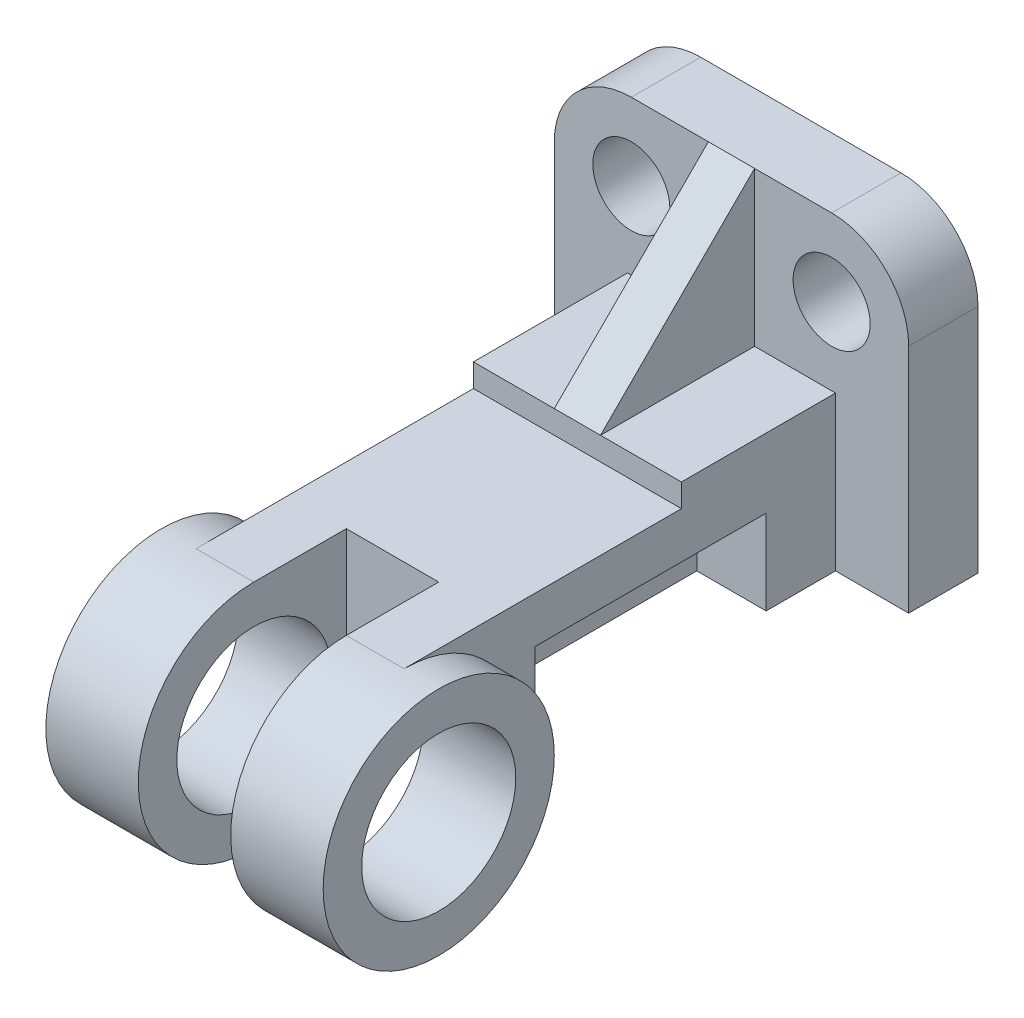
ISO-10303-21;
HEADER;
FILE_DESCRIPTION(('STEP AP214'),'2;1');
FILE_NAME('part.step','',(''),(''),'','','');
FILE_SCHEMA(('AUTOMOTIVE_DESIGN { 1 0 10303 214 1 1 1 1 }'));
ENDSEC;
DATA;
#1=APPLICATION_CONTEXT('core data for automotive mechanical design processes');
#2=APPLICATION_PROTOCOL_DEFINITION('international standard','automotive_design',2000,#1);
#3=PRODUCT_CONTEXT('',#1,'mechanical');
#4=PRODUCT('Part','Part','',(#3));
#5=PRODUCT_RELATED_PRODUCT_CATEGORY('part','',(#4));
#6=PRODUCT_DEFINITION_FORMATION('','',#4);
#7=PRODUCT_DEFINITION_CONTEXT('part definition',#1,'design');
#8=PRODUCT_DEFINITION('design','',#6,#7);
#9=PRODUCT_DEFINITION_SHAPE('','',#8);
#10=(LENGTH_UNIT() NAMED_UNIT(*) SI_UNIT(.MILLI.,.METRE.));
#11=(NAMED_UNIT(*) PLANE_ANGLE_UNIT() SI_UNIT($,.RADIAN.));
#12=(NAMED_UNIT(*) SI_UNIT($,.STERADIAN.) SOLID_ANGLE_UNIT());
#13=UNCERTAINTY_MEASURE_WITH_UNIT(LENGTH_MEASURE(1.E-05),#10,'distance_accuracy_value','');
#14=(GEOMETRIC_REPRESENTATION_CONTEXT(3) GLOBAL_UNCERTAINTY_ASSIGNED_CONTEXT((#13)) GLOBAL_UNIT_ASSIGNED_CONTEXT((#10,
#11,#12)) REPRESENTATION_CONTEXT('',''));
#15=CARTESIAN_POINT('',(0.,0.,0.));
#16=DIRECTION('',(0.,0.,1.));
#17=DIRECTION('',(1.,0.,0.));
#18=AXIS2_PLACEMENT_3D('',#15,#16,#17);
#19=CARTESIAN_POINT('',(0.,0.,106.));
#20=DIRECTION('',(0.,0.,1.));
#21=DIRECTION('',(1.,0.,0.));
#22=AXIS2_PLACEMENT_3D('',#19,#20,#21);
#23=PLANE('',#22);
#24=DIRECTION('',(1.,0.,0.));
#25=VECTOR('',#24,1.);
#26=CARTESIAN_POINT('',(0.,34.,106.));
#27=LINE('',#26,#25);
#28=CARTESIAN_POINT('',(34.,34.,106.));
#29=VERTEX_POINT('',#28);
#30=CARTESIAN_POINT('',(58.,34.,106.));
#31=VERTEX_POINT('',#30);
#32=EDGE_CURVE('E66',#29,#31,#27,.T.);
#33=ORIENTED_EDGE('',*,*,#32,.F.);
#34=DIRECTION('',(0.,-1.,0.));
#35=VECTOR('',#34,1.);
#36=CARTESIAN_POINT('',(34.,0.,106.));
#37=LINE('',#36,#35);
#38=CARTESIAN_POINT('',(34.,0.,106.));
#39=VERTEX_POINT('',#38);
#40=EDGE_CURVE('E256',#29,#39,#37,.T.);
#41=ORIENTED_EDGE('',*,*,#40,.T.);
#42=DIRECTION('',(1.,0.,0.));
#43=VECTOR('',#42,1.);
#44=CARTESIAN_POINT('',(0.,0.,106.));
#45=LINE('',#44,#43);
#46=CARTESIAN_POINT('',(58.,0.,106.));
#47=VERTEX_POINT('',#46);
#48=EDGE_CURVE('E355',#39,#47,#45,.T.);
#49=ORIENTED_EDGE('',*,*,#48,.T.);
#50=DIRECTION('',(0.,1.,0.));
#51=VECTOR('',#50,1.);
#52=CARTESIAN_POINT('',(58.,0.,106.));
#53=LINE('',#52,#51);
#54=EDGE_CURVE('E245',#47,#31,#53,.T.);
#55=ORIENTED_EDGE('',*,*,#54,.T.);
#56=EDGE_LOOP('',(#33,#41,#49,#55));
#57=FACE_BOUND('',#56,.T.);
#58=ADVANCED_FACE('F43',(#57),#23,.T.);
#59=CARTESIAN_POINT('',(10.,4.00000000000001,130.));
#60=DIRECTION('',(1.,0.,0.));
#61=DIRECTION('',(0.,0.,-1.));
#62=AXIS2_PLACEMENT_3D('',#59,#60,#61);
#63=CYLINDRICAL_SURFACE('',#62,30.);
#64=CARTESIAN_POINT('',(10.,4.00000000000001,130.));
#65=DIRECTION('',(1.,0.,0.));
#66=DIRECTION('',(0.,0.,-1.));
#67=AXIS2_PLACEMENT_3D('',#64,#65,#66);
#68=CIRCLE('',#67,30.);
#69=CARTESIAN_POINT('',(10.,4.00000000000001,100.));
#70=VERTEX_POINT('',#69);
#71=EDGE_CURVE('E251',#70,#70,#68,.T.);
#72=ORIENTED_EDGE('',*,*,#71,.T.);
#73=EDGE_LOOP('',(#72));
#74=FACE_BOUND('',#73,.T.);
#75=CARTESIAN_POINT('',(34.,4.00000000000001,130.));
#76=DIRECTION('',(1.,0.,0.));
#77=DIRECTION('',(0.,0.,-1.));
#78=AXIS2_PLACEMENT_3D('',#75,#76,#77);
#79=CIRCLE('',#78,30.);
#80=CARTESIAN_POINT('',(34.,34.,130.));
#81=VERTEX_POINT('',#80);
#82=CARTESIAN_POINT('',(34.,0.,100.267862505363));
#83=VERTEX_POINT('',#82);
#84=EDGE_CURVE('E242',#81,#83,#79,.T.);
#85=ORIENTED_EDGE('',*,*,#84,.F.);
#86=DIRECTION('',(1.,0.,0.));
#87=VECTOR('',#86,1.);
#88=CARTESIAN_POINT('',(19.,34.,130.));
#89=LINE('',#88,#87);
#90=CARTESIAN_POINT('',(19.,34.,130.));
#91=VERTEX_POINT('',#90);
#92=EDGE_CURVE('E228',#91,#81,#89,.T.);
#93=ORIENTED_EDGE('',*,*,#92,.F.);
#94=CARTESIAN_POINT('',(19.,4.00000000000001,130.));
#95=DIRECTION('',(1.,0.,0.));
#96=DIRECTION('',(0.,0.,-1.));
#97=AXIS2_PLACEMENT_3D('',#94,#95,#96);
#98=CIRCLE('',#97,30.);
#99=CARTESIAN_POINT('',(19.,0.,100.267862505363));
#100=VERTEX_POINT('',#99);
#101=EDGE_CURVE('E55',#100,#91,#98,.T.);
#102=ORIENTED_EDGE('',*,*,#101,.F.);
#103=DIRECTION('',(1.,0.,0.));
#104=VECTOR('',#103,1.);
#105=CARTESIAN_POINT('',(10.,0.,100.267862505363));
#106=LINE('',#105,#104);
#107=EDGE_CURVE('E258',#83,#100,#106,.F.);
#108=ORIENTED_EDGE('',*,*,#107,.F.);
#109=EDGE_LOOP('',(#85,#93,#102,#108));
#110=FACE_BOUND('',#109,.T.);
#111=ADVANCED_FACE('F243',(#74,#110),#63,.T.);
#112=CARTESIAN_POINT('',(0.,0.,18.));
#113=DIRECTION('',(0.,1.,0.));
#114=DIRECTION('',(0.,0.,1.));
#115=AXIS2_PLACEMENT_3D('',#112,#113,#114);
#116=PLANE('',#115);
#117=DIRECTION('',(0.,0.,1.));
#118=VECTOR('',#117,1.);
#119=CARTESIAN_POINT('',(34.,0.,18.));
#120=LINE('',#119,#118);
#121=EDGE_CURVE('E11',#83,#39,#120,.T.);
#122=ORIENTED_EDGE('',*,*,#121,.F.);
#123=ORIENTED_EDGE('',*,*,#107,.T.);
#124=DIRECTION('',(0.,0.,-1.));
#125=VECTOR('',#124,1.);
#126=CARTESIAN_POINT('',(19.,0.,106.));
#127=LINE('',#126,#125);
#128=CARTESIAN_POINT('',(19.,0.,96.));
#129=VERTEX_POINT('',#128);
#130=EDGE_CURVE('E238',#100,#129,#127,.T.);
#131=ORIENTED_EDGE('',*,*,#130,.T.);
#132=DIRECTION('',(-1.,0.,0.));
#133=VECTOR('',#132,1.);
#134=CARTESIAN_POINT('',(37.,0.,96.));
#135=LINE('',#134,#133);
#136=CARTESIAN_POINT('',(37.,0.,96.));
#137=VERTEX_POINT('',#136);
#138=EDGE_CURVE('E304',#137,#129,#135,.T.);
#139=ORIENTED_EDGE('',*,*,#138,.F.);
#140=DIRECTION('',(0.,0.,1.));
#141=VECTOR('',#140,1.);
#142=CARTESIAN_POINT('',(37.,0.,0.));
#143=LINE('',#142,#141);
#144=CARTESIAN_POINT('',(37.,0.,36.));
#145=VERTEX_POINT('',#144);
#146=EDGE_CURVE('E294',#145,#137,#143,.T.);
#147=ORIENTED_EDGE('',*,*,#146,.F.);
#148=DIRECTION('',(-1.,0.,0.));
#149=VECTOR('',#148,1.);
#150=CARTESIAN_POINT('',(37.,0.,36.));
#151=LINE('',#150,#149);
#152=CARTESIAN_POINT('',(19.,0.,36.));
#153=VERTEX_POINT('',#152);
#154=EDGE_CURVE('E307',#145,#153,#151,.T.);
#155=ORIENTED_EDGE('',*,*,#154,.T.);
#156=CARTESIAN_POINT('',(19.,0.,18.));
#157=VERTEX_POINT('',#156);
#158=EDGE_CURVE('E351',#153,#157,#127,.T.);
#159=ORIENTED_EDGE('',*,*,#158,.T.);
#160=DIRECTION('',(1.,0.,0.));
#161=VECTOR('',#160,1.);
#162=CARTESIAN_POINT('',(0.,0.,18.));
#163=LINE('',#162,#161);
#164=CARTESIAN_POINT('',(0.,0.,18.));
#165=VERTEX_POINT('',#164);
#166=EDGE_CURVE('E401',#165,#157,#163,.T.);
#167=ORIENTED_EDGE('',*,*,#166,.F.);
#168=DIRECTION('',(0.,0.,-1.));
#169=VECTOR('',#168,1.);
#170=CARTESIAN_POINT('',(0.,0.,18.));
#171=LINE('',#170,#169);
#172=CARTESIAN_POINT('',(0.,0.,0.));
#173=VERTEX_POINT('',#172);
#174=EDGE_CURVE('E425',#165,#173,#171,.T.);
#175=ORIENTED_EDGE('',*,*,#174,.T.);
#176=DIRECTION('',(1.,0.,0.));
#177=VECTOR('',#176,1.);
#178=CARTESIAN_POINT('',(0.,0.,0.));
#179=LINE('',#178,#177);
#180=CARTESIAN_POINT('',(92.,0.,0.));
#181=VERTEX_POINT('',#180);
#182=EDGE_CURVE('E414',#173,#181,#179,.T.);
#183=ORIENTED_EDGE('',*,*,#182,.T.);
#184=DIRECTION('',(0.,0.,-1.));
#185=VECTOR('',#184,1.);
#186=CARTESIAN_POINT('',(92.,0.,18.));
#187=LINE('',#186,#185);
#188=CARTESIAN_POINT('',(92.,0.,18.));
#189=VERTEX_POINT('',#188);
#190=EDGE_CURVE('E413',#189,#181,#187,.T.);
#191=ORIENTED_EDGE('',*,*,#190,.F.);
#192=CARTESIAN_POINT('',(73.,0.,18.));
#193=VERTEX_POINT('',#192);
#194=EDGE_CURVE('E402',#193,#189,#163,.T.);
#195=ORIENTED_EDGE('',*,*,#194,.F.);
#196=DIRECTION('',(0.,0.,-1.));
#197=VECTOR('',#196,1.);
#198=CARTESIAN_POINT('',(73.,0.,106.));
#199=LINE('',#198,#197);
#200=CARTESIAN_POINT('',(73.,0.,36.));
#201=VERTEX_POINT('',#200);
#202=EDGE_CURVE('E367',#201,#193,#199,.T.);
#203=ORIENTED_EDGE('',*,*,#202,.F.);
#204=DIRECTION('',(1.,0.,0.));
#205=VECTOR('',#204,1.);
#206=CARTESIAN_POINT('',(55.,0.,36.));
#207=LINE('',#206,#205);
#208=CARTESIAN_POINT('',(55.,0.,36.));
#209=VERTEX_POINT('',#208);
#210=EDGE_CURVE('E341',#209,#201,#207,.T.);
#211=ORIENTED_EDGE('',*,*,#210,.F.);
#212=DIRECTION('',(0.,0.,-1.));
#213=VECTOR('',#212,1.);
#214=CARTESIAN_POINT('',(55.,0.,0.));
#215=LINE('',#214,#213);
#216=CARTESIAN_POINT('',(55.,0.,96.));
#217=VERTEX_POINT('',#216);
#218=EDGE_CURVE('E329',#217,#209,#215,.T.);
#219=ORIENTED_EDGE('',*,*,#218,.F.);
#220=DIRECTION('',(1.,0.,0.));
#221=VECTOR('',#220,1.);
#222=CARTESIAN_POINT('',(55.,0.,96.));
#223=LINE('',#222,#221);
#224=CARTESIAN_POINT('',(73.,0.,96.));
#225=VERTEX_POINT('',#224);
#226=EDGE_CURVE('E350',#217,#225,#223,.T.);
#227=ORIENTED_EDGE('',*,*,#226,.T.);
#228=CARTESIAN_POINT('',(73.,0.,100.267862505363));
#229=VERTEX_POINT('',#228);
#230=EDGE_CURVE('E369',#229,#225,#199,.T.);
#231=ORIENTED_EDGE('',*,*,#230,.F.);
#232=DIRECTION('',(-1.,0.,0.));
#233=VECTOR('',#232,1.);
#234=CARTESIAN_POINT('',(82.,0.,100.267862505363));
#235=LINE('',#234,#233);
#236=CARTESIAN_POINT('',(58.,0.,100.267862505363));
#237=VERTEX_POINT('',#236);
#238=EDGE_CURVE('E284',#237,#229,#235,.F.);
#239=ORIENTED_EDGE('',*,*,#238,.F.);
#240=DIRECTION('',(0.,0.,-1.));
#241=VECTOR('',#240,1.);
#242=CARTESIAN_POINT('',(58.,0.,18.));
#243=LINE('',#242,#241);
#244=EDGE_CURVE('E278',#47,#237,#243,.T.);
#245=ORIENTED_EDGE('',*,*,#244,.F.);
#246=ORIENTED_EDGE('',*,*,#48,.F.);
#247=EDGE_LOOP('',(#122,#123,#131,#139,#147,#155,#159,#167,#175,#183,#191,#195,#203,#211,#219,
#227,#231,#239,#245,#246));
#248=FACE_BOUND('',#247,.T.);
#249=ADVANCED_FACE('F471',(#248),#116,.F.);
#250=CARTESIAN_POINT('',(19.,0.,106.));
#251=DIRECTION('',(1.,0.,0.));
#252=DIRECTION('',(0.,0.,-1.));
#253=AXIS2_PLACEMENT_3D('',#250,#251,#252);
#254=PLANE('',#253);
#255=ORIENTED_EDGE('',*,*,#130,.F.);
#256=ORIENTED_EDGE('',*,*,#101,.T.);
#257=DIRECTION('',(0.,0.,-1.));
#258=VECTOR('',#257,1.);
#259=CARTESIAN_POINT('',(19.,34.,106.));
#260=LINE('',#259,#258);
#261=CARTESIAN_POINT('',(19.,34.,58.));
#262=VERTEX_POINT('',#261);
#263=EDGE_CURVE('E225',#91,#262,#260,.T.);
#264=ORIENTED_EDGE('',*,*,#263,.T.);
#265=DIRECTION('',(0.,1.,0.));
#266=VECTOR('',#265,1.);
#267=CARTESIAN_POINT('',(19.,0.,58.));
#268=LINE('',#267,#266);
#269=CARTESIAN_POINT('',(19.,40.,58.));
#270=VERTEX_POINT('',#269);
#271=EDGE_CURVE('E455',#262,#270,#268,.T.);
#272=ORIENTED_EDGE('',*,*,#271,.T.);
#273=DIRECTION('',(0.,0.,-1.));
#274=VECTOR('',#273,1.);
#275=CARTESIAN_POINT('',(19.,40.,106.));
#276=LINE('',#275,#274);
#277=CARTESIAN_POINT('',(19.,40.,18.));
#278=VERTEX_POINT('',#277);
#279=EDGE_CURVE('E362',#270,#278,#276,.T.);
#280=ORIENTED_EDGE('',*,*,#279,.T.);
#281=DIRECTION('',(0.,-1.,0.));
#282=VECTOR('',#281,1.);
#283=CARTESIAN_POINT('',(19.,0.,18.));
#284=LINE('',#283,#282);
#285=EDGE_CURVE('E353',#278,#157,#284,.T.);
#286=ORIENTED_EDGE('',*,*,#285,.T.);
#287=ORIENTED_EDGE('',*,*,#158,.F.);
#288=DIRECTION('',(0.,1.,0.));
#289=VECTOR('',#288,1.);
#290=CARTESIAN_POINT('',(19.,0.,36.));
#291=LINE('',#290,#289);
#292=CARTESIAN_POINT('',(19.,22.,36.));
#293=VERTEX_POINT('',#292);
#294=EDGE_CURVE('E293',#153,#293,#291,.T.);
#295=ORIENTED_EDGE('',*,*,#294,.T.);
#296=DIRECTION('',(0.,0.,1.));
#297=VECTOR('',#296,1.);
#298=CARTESIAN_POINT('',(19.,22.,0.));
#299=LINE('',#298,#297);
#300=CARTESIAN_POINT('',(19.,22.,96.));
#301=VERTEX_POINT('',#300);
#302=EDGE_CURVE('E297',#293,#301,#299,.T.);
#303=ORIENTED_EDGE('',*,*,#302,.T.);
#304=DIRECTION('',(0.,-1.,0.));
#305=VECTOR('',#304,1.);
#306=CARTESIAN_POINT('',(19.,0.,96.));
#307=LINE('',#306,#305);
#308=EDGE_CURVE('E290',#301,#129,#307,.T.);
#309=ORIENTED_EDGE('',*,*,#308,.T.);
#310=EDGE_LOOP('',(#255,#256,#264,#272,#280,#286,#287,#295,#303,#309));
#311=FACE_BOUND('',#310,.T.);
#312=ADVANCED_FACE('F236',(#311),#254,.F.);
#313=CARTESIAN_POINT('',(0.,40.,106.));
#314=DIRECTION('',(0.,1.,0.));
#315=DIRECTION('',(0.,0.,1.));
#316=AXIS2_PLACEMENT_3D('',#313,#314,#315);
#317=PLANE('',#316);
#318=DIRECTION('',(1.,0.,0.));
#319=VECTOR('',#318,1.);
#320=CARTESIAN_POINT('',(0.,40.,58.));
#321=LINE('',#320,#319);
#322=CARTESIAN_POINT('',(52.,40.,58.));
#323=VERTEX_POINT('',#322);
#324=CARTESIAN_POINT('',(73.,40.,58.));
#325=VERTEX_POINT('',#324);
#326=EDGE_CURVE('E316',#323,#325,#321,.T.);
#327=ORIENTED_EDGE('',*,*,#326,.T.);
#328=DIRECTION('',(0.,0.,-1.));
#329=VECTOR('',#328,1.);
#330=CARTESIAN_POINT('',(73.,40.,106.));
#331=LINE('',#330,#329);
#332=CARTESIAN_POINT('',(73.,40.,18.));
#333=VERTEX_POINT('',#332);
#334=EDGE_CURVE('E370',#325,#333,#331,.T.);
#335=ORIENTED_EDGE('',*,*,#334,.T.);
#336=DIRECTION('',(1.,0.,0.));
#337=VECTOR('',#336,1.);
#338=CARTESIAN_POINT('',(0.,40.,18.));
#339=LINE('',#338,#337);
#340=CARTESIAN_POINT('',(52.,40.,18.));
#341=VERTEX_POINT('',#340);
#342=EDGE_CURVE('E356',#341,#333,#339,.T.);
#343=ORIENTED_EDGE('',*,*,#342,.F.);
#344=DIRECTION('',(0.,0.,-1.));
#345=VECTOR('',#344,1.);
#346=CARTESIAN_POINT('',(52.,40.,58.));
#347=LINE('',#346,#345);
#348=EDGE_CURVE('E384',#323,#341,#347,.T.);
#349=ORIENTED_EDGE('',*,*,#348,.F.);
#350=EDGE_LOOP('',(#327,#335,#343,#349));
#351=FACE_BOUND('',#350,.T.);
#352=ADVANCED_FACE('F505',(#351),#317,.T.);
#353=CARTESIAN_POINT('',(0.,0.,18.));
#354=DIRECTION('',(0.,0.,1.));
#355=DIRECTION('',(1.,0.,0.));
#356=AXIS2_PLACEMENT_3D('',#353,#354,#355);
#357=PLANE('',#356);
#358=CARTESIAN_POINT('',(72.,60.,18.));
#359=DIRECTION('',(0.,0.,1.));
#360=DIRECTION('',(1.,0.,0.));
#361=AXIS2_PLACEMENT_3D('',#358,#359,#360);
#362=CIRCLE('',#361,9.99999999999999);
#363=CARTESIAN_POINT('',(82.,60.,18.));
#364=VERTEX_POINT('',#363);
#365=EDGE_CURVE('E391',#364,#364,#362,.T.);
#366=ORIENTED_EDGE('',*,*,#365,.F.);
#367=EDGE_LOOP('',(#366));
#368=FACE_BOUND('',#367,.T.);
#369=ORIENTED_EDGE('',*,*,#342,.T.);
#370=DIRECTION('',(0.,1.,0.));
#371=VECTOR('',#370,1.);
#372=CARTESIAN_POINT('',(73.,0.,18.));
#373=LINE('',#372,#371);
#374=EDGE_CURVE('E345',#193,#333,#373,.T.);
#375=ORIENTED_EDGE('',*,*,#374,.F.);
#376=ORIENTED_EDGE('',*,*,#194,.T.);
#377=DIRECTION('',(0.,1.,0.));
#378=VECTOR('',#377,1.);
#379=CARTESIAN_POINT('',(92.,0.,18.));
#380=LINE('',#379,#378);
#381=CARTESIAN_POINT('',(92.,60.,18.));
#382=VERTEX_POINT('',#381);
#383=EDGE_CURVE('E408',#189,#382,#380,.T.);
#384=ORIENTED_EDGE('',*,*,#383,.T.);
#385=CARTESIAN_POINT('',(72.,60.,18.));
#386=DIRECTION('',(0.,0.,1.));
#387=DIRECTION('',(1.,0.,0.));
#388=AXIS2_PLACEMENT_3D('',#385,#386,#387);
#389=CIRCLE('',#388,20.);
#390=CARTESIAN_POINT('',(72.,80.,18.));
#391=VERTEX_POINT('',#390);
#392=EDGE_CURVE('E439',#382,#391,#389,.T.);
#393=ORIENTED_EDGE('',*,*,#392,.T.);
#394=DIRECTION('',(-1.,0.,0.));
#395=VECTOR('',#394,1.);
#396=CARTESIAN_POINT('',(92.,80.,18.));
#397=LINE('',#396,#395);
#398=CARTESIAN_POINT('',(52.,80.,18.));
#399=VERTEX_POINT('',#398);
#400=EDGE_CURVE('E406',#391,#399,#397,.T.);
#401=ORIENTED_EDGE('',*,*,#400,.T.);
#402=DIRECTION('',(0.,1.,0.));
#403=VECTOR('',#402,1.);
#404=CARTESIAN_POINT('',(52.,0.,18.));
#405=LINE('',#404,#403);
#406=EDGE_CURVE('E375',#341,#399,#405,.T.);
#407=ORIENTED_EDGE('',*,*,#406,.F.);
#408=EDGE_LOOP('',(#369,#375,#376,#384,#393,#401,#407));
#409=FACE_BOUND('',#408,.T.);
#410=ADVANCED_FACE('F500',(#368,#409),#357,.T.);
#411=CARTESIAN_POINT('',(0.,80.,18.));
#412=DIRECTION('',(1.,0.,0.));
#413=DIRECTION('',(0.,0.,-1.));
#414=AXIS2_PLACEMENT_3D('',#411,#412,#413);
#415=PLANE('',#414);
#416=DIRECTION('',(0.,-1.,0.));
#417=VECTOR('',#416,1.);
#418=CARTESIAN_POINT('',(0.,80.,18.));
#419=LINE('',#418,#417);
#420=CARTESIAN_POINT('',(0.,60.,18.));
#421=VERTEX_POINT('',#420);
#422=EDGE_CURVE('E396',#421,#165,#419,.T.);
#423=ORIENTED_EDGE('',*,*,#422,.F.);
#424=DIRECTION('',(0.,0.,-1.));
#425=VECTOR('',#424,1.);
#426=CARTESIAN_POINT('',(0.,60.,18.));
#427=LINE('',#426,#425);
#428=CARTESIAN_POINT('',(0.,60.,0.));
#429=VERTEX_POINT('',#428);
#430=EDGE_CURVE('E430',#421,#429,#427,.T.);
#431=ORIENTED_EDGE('',*,*,#430,.T.);
#432=DIRECTION('',(0.,-1.,0.));
#433=VECTOR('',#432,1.);
#434=CARTESIAN_POINT('',(0.,80.,0.));
#435=LINE('',#434,#433);
#436=EDGE_CURVE('E386',#429,#173,#435,.T.);
#437=ORIENTED_EDGE('',*,*,#436,.T.);
#438=ORIENTED_EDGE('',*,*,#174,.F.);
#439=EDGE_LOOP('',(#423,#431,#437,#438));
#440=FACE_BOUND('',#439,.T.);
#441=ADVANCED_FACE('F610',(#440),#415,.F.);
#442=CARTESIAN_POINT('',(92.,0.,18.));
#443=DIRECTION('',(-1.,0.,0.));
#444=DIRECTION('',(0.,0.,1.));
#445=AXIS2_PLACEMENT_3D('',#442,#443,#444);
#446=PLANE('',#445);
#447=DIRECTION('',(0.,1.,0.));
#448=VECTOR('',#447,1.);
#449=CARTESIAN_POINT('',(92.,0.,0.));
#450=LINE('',#449,#448);
#451=CARTESIAN_POINT('',(92.,60.,0.));
#452=VERTEX_POINT('',#451);
#453=EDGE_CURVE('E420',#181,#452,#450,.T.);
#454=ORIENTED_EDGE('',*,*,#453,.T.);
#455=DIRECTION('',(0.,0.,-1.));
#456=VECTOR('',#455,1.);
#457=CARTESIAN_POINT('',(92.,60.,18.));
#458=LINE('',#457,#456);
#459=EDGE_CURVE('E443',#452,#382,#458,.F.);
#460=ORIENTED_EDGE('',*,*,#459,.T.);
#461=ORIENTED_EDGE('',*,*,#383,.F.);
#462=ORIENTED_EDGE('',*,*,#190,.T.);
#463=EDGE_LOOP('',(#454,#460,#461,#462));
#464=FACE_BOUND('',#463,.T.);
#465=ADVANCED_FACE('F602',(#464),#446,.F.);
#466=CARTESIAN_POINT('',(92.,80.,18.));
#467=DIRECTION('',(0.,-1.,0.));
#468=DIRECTION('',(0.,0.,-1.));
#469=AXIS2_PLACEMENT_3D('',#466,#467,#468);
#470=PLANE('',#469);
#471=CARTESIAN_POINT('',(40.,80.,18.));
#472=VERTEX_POINT('',#471);
#473=CARTESIAN_POINT('',(20.,80.,18.));
#474=VERTEX_POINT('',#473);
#475=EDGE_CURVE('E410',#472,#474,#397,.T.);
#476=ORIENTED_EDGE('',*,*,#475,.F.);
#477=DIRECTION('',(1.,0.,0.));
#478=VECTOR('',#477,1.);
#479=CARTESIAN_POINT('',(52.,80.,18.));
#480=LINE('',#479,#478);
#481=EDGE_CURVE('E449',#472,#399,#480,.T.);
#482=ORIENTED_EDGE('',*,*,#481,.T.);
#483=ORIENTED_EDGE('',*,*,#400,.F.);
#484=DIRECTION('',(0.,0.,-1.));
#485=VECTOR('',#484,1.);
#486=CARTESIAN_POINT('',(72.,80.,18.));
#487=LINE('',#486,#485);
#488=CARTESIAN_POINT('',(72.,80.,0.));
#489=VERTEX_POINT('',#488);
#490=EDGE_CURVE('E432',#391,#489,#487,.T.);
#491=ORIENTED_EDGE('',*,*,#490,.T.);
#492=DIRECTION('',(-1.,0.,0.));
#493=VECTOR('',#492,1.);
#494=CARTESIAN_POINT('',(92.,80.,0.));
#495=LINE('',#494,#493);
#496=CARTESIAN_POINT('',(20.,80.,0.));
#497=VERTEX_POINT('',#496);
#498=EDGE_CURVE('E405',#489,#497,#495,.T.);
#499=ORIENTED_EDGE('',*,*,#498,.T.);
#500=DIRECTION('',(0.,0.,-1.));
#501=VECTOR('',#500,1.);
#502=CARTESIAN_POINT('',(20.,80.,18.));
#503=LINE('',#502,#501);
#504=EDGE_CURVE('E440',#497,#474,#503,.F.);
#505=ORIENTED_EDGE('',*,*,#504,.T.);
#506=EDGE_LOOP('',(#476,#482,#483,#491,#499,#505));
#507=FACE_BOUND('',#506,.T.);
#508=ADVANCED_FACE('F597',(#507),#470,.F.);
#509=CARTESIAN_POINT('',(40.,40.,18.));
#510=VERTEX_POINT('',#509);
#511=EDGE_CURVE('E360',#278,#510,#339,.T.);
#512=ORIENTED_EDGE('',*,*,#511,.T.);
#513=DIRECTION('',(0.,-1.,0.));
#514=VECTOR('',#513,1.);
#515=CARTESIAN_POINT('',(40.,0.,18.));
#516=LINE('',#515,#514);
#517=EDGE_CURVE('E380',#472,#510,#516,.T.);
#518=ORIENTED_EDGE('',*,*,#517,.F.);
#519=ORIENTED_EDGE('',*,*,#475,.T.);
#520=CARTESIAN_POINT('',(20.,60.,18.));
#521=DIRECTION('',(0.,0.,1.));
#522=DIRECTION('',(1.,0.,0.));
#523=AXIS2_PLACEMENT_3D('',#520,#521,#522);
#524=CIRCLE('',#523,20.);
#525=EDGE_CURVE('E445',#474,#421,#524,.T.);
#526=ORIENTED_EDGE('',*,*,#525,.T.);
#527=ORIENTED_EDGE('',*,*,#422,.T.);
#528=ORIENTED_EDGE('',*,*,#166,.T.);
#529=ORIENTED_EDGE('',*,*,#285,.F.);
#530=EDGE_LOOP('',(#512,#518,#519,#526,#527,#528,#529));
#531=FACE_BOUND('',#530,.T.);
#532=CARTESIAN_POINT('',(20.,60.,18.));
#533=DIRECTION('',(0.,0.,1.));
#534=DIRECTION('',(1.,0.,0.));
#535=AXIS2_PLACEMENT_3D('',#532,#533,#534);
#536=CIRCLE('',#535,10.);
#537=CARTESIAN_POINT('',(30.,60.,18.));
#538=VERTEX_POINT('',#537);
#539=EDGE_CURVE('E388',#538,#538,#536,.T.);
#540=ORIENTED_EDGE('',*,*,#539,.F.);
#541=EDGE_LOOP('',(#540));
#542=FACE_BOUND('',#541,.T.);
#543=ADVANCED_FACE('F518',(#531,#542),#357,.T.);
#544=CARTESIAN_POINT('',(0.,0.,0.));
#545=DIRECTION('',(0.,0.,1.));
#546=DIRECTION('',(1.,0.,0.));
#547=AXIS2_PLACEMENT_3D('',#544,#545,#546);
#548=PLANE('',#547);
#549=CARTESIAN_POINT('',(72.,60.,0.));
#550=DIRECTION('',(0.,0.,1.));
#551=DIRECTION('',(1.,0.,0.));
#552=AXIS2_PLACEMENT_3D('',#549,#550,#551);
#553=CIRCLE('',#552,9.99999999999999);
#554=CARTESIAN_POINT('',(82.,60.,0.));
#555=VERTEX_POINT('',#554);
#556=EDGE_CURVE('E389',#555,#555,#553,.T.);
#557=ORIENTED_EDGE('',*,*,#556,.T.);
#558=EDGE_LOOP('',(#557));
#559=FACE_BOUND('',#558,.T.);
#560=CARTESIAN_POINT('',(20.,60.,0.));
#561=DIRECTION('',(0.,0.,1.));
#562=DIRECTION('',(1.,0.,0.));
#563=AXIS2_PLACEMENT_3D('',#560,#561,#562);
#564=CIRCLE('',#563,10.);
#565=CARTESIAN_POINT('',(30.,60.,0.));
#566=VERTEX_POINT('',#565);
#567=EDGE_CURVE('E392',#566,#566,#564,.T.);
#568=ORIENTED_EDGE('',*,*,#567,.T.);
#569=EDGE_LOOP('',(#568));
#570=FACE_BOUND('',#569,.T.);
#571=ORIENTED_EDGE('',*,*,#436,.F.);
#572=CARTESIAN_POINT('',(20.,60.,0.));
#573=DIRECTION('',(0.,0.,1.));
#574=DIRECTION('',(1.,0.,0.));
#575=AXIS2_PLACEMENT_3D('',#572,#573,#574);
#576=CIRCLE('',#575,20.);
#577=EDGE_CURVE('E435',#429,#497,#576,.F.);
#578=ORIENTED_EDGE('',*,*,#577,.T.);
#579=ORIENTED_EDGE('',*,*,#498,.F.);
#580=CARTESIAN_POINT('',(72.,60.,0.));
#581=DIRECTION('',(0.,0.,1.));
#582=DIRECTION('',(1.,0.,0.));
#583=AXIS2_PLACEMENT_3D('',#580,#581,#582);
#584=CIRCLE('',#583,20.);
#585=EDGE_CURVE('E427',#489,#452,#584,.F.);
#586=ORIENTED_EDGE('',*,*,#585,.T.);
#587=ORIENTED_EDGE('',*,*,#453,.F.);
#588=ORIENTED_EDGE('',*,*,#182,.F.);
#589=EDGE_LOOP('',(#571,#578,#579,#586,#587,#588));
#590=FACE_BOUND('',#589,.T.);
#591=ADVANCED_FACE('F593',(#559,#570,#590),#548,.F.);
#592=CARTESIAN_POINT('',(20.,60.,18.));
#593=DIRECTION('',(0.,0.,-1.));
#594=DIRECTION('',(-1.,0.,0.));
#595=AXIS2_PLACEMENT_3D('',#592,#593,#594);
#596=CYLINDRICAL_SURFACE('',#595,20.);
#597=ORIENTED_EDGE('',*,*,#525,.F.);
#598=ORIENTED_EDGE('',*,*,#504,.F.);
#599=ORIENTED_EDGE('',*,*,#577,.F.);
#600=ORIENTED_EDGE('',*,*,#430,.F.);
#601=EDGE_LOOP('',(#597,#598,#599,#600));
#602=FACE_BOUND('',#601,.T.);
#603=ADVANCED_FACE('F599',(#602),#596,.T.);
#604=CARTESIAN_POINT('',(72.,60.,18.));
#605=DIRECTION('',(0.,0.,-1.));
#606=DIRECTION('',(-1.,0.,0.));
#607=AXIS2_PLACEMENT_3D('',#604,#605,#606);
#608=CYLINDRICAL_SURFACE('',#607,20.);
#609=ORIENTED_EDGE('',*,*,#392,.F.);
#610=ORIENTED_EDGE('',*,*,#459,.F.);
#611=ORIENTED_EDGE('',*,*,#585,.F.);
#612=ORIENTED_EDGE('',*,*,#490,.F.);
#613=EDGE_LOOP('',(#609,#610,#611,#612));
#614=FACE_BOUND('',#613,.T.);
#615=ADVANCED_FACE('F592',(#614),#608,.T.);
#616=CARTESIAN_POINT('',(20.,60.,0.));
#617=DIRECTION('',(0.,0.,1.));
#618=DIRECTION('',(1.,0.,0.));
#619=AXIS2_PLACEMENT_3D('',#616,#617,#618);
#620=CYLINDRICAL_SURFACE('',#619,10.);
#621=ORIENTED_EDGE('',*,*,#567,.F.);
#622=EDGE_LOOP('',(#621));
#623=FACE_BOUND('',#622,.T.);
#624=ORIENTED_EDGE('',*,*,#539,.T.);
#625=EDGE_LOOP('',(#624));
#626=FACE_BOUND('',#625,.T.);
#627=ADVANCED_FACE('F590',(#623,#626),#620,.F.);
#628=CARTESIAN_POINT('',(72.,60.,0.));
#629=DIRECTION('',(0.,0.,1.));
#630=DIRECTION('',(1.,0.,0.));
#631=AXIS2_PLACEMENT_3D('',#628,#629,#630);
#632=CYLINDRICAL_SURFACE('',#631,9.99999999999999);
#633=ORIENTED_EDGE('',*,*,#556,.F.);
#634=EDGE_LOOP('',(#633));
#635=FACE_BOUND('',#634,.T.);
#636=ORIENTED_EDGE('',*,*,#365,.T.);
#637=EDGE_LOOP('',(#636));
#638=FACE_BOUND('',#637,.T.);
#639=ADVANCED_FACE('F582',(#635,#638),#632,.F.);
#640=CARTESIAN_POINT('',(52.,0.,58.));
#641=DIRECTION('',(-1.,0.,0.));
#642=DIRECTION('',(0.,0.,1.));
#643=AXIS2_PLACEMENT_3D('',#640,#641,#642);
#644=PLANE('',#643);
#645=ORIENTED_EDGE('',*,*,#406,.T.);
#646=DIRECTION('',(0.,-0.707106781186548,0.707106781186548));
#647=VECTOR('',#646,1.);
#648=CARTESIAN_POINT('',(52.,40.,58.));
#649=LINE('',#648,#647);
#650=EDGE_CURVE('E448',#399,#323,#649,.T.);
#651=ORIENTED_EDGE('',*,*,#650,.T.);
#652=ORIENTED_EDGE('',*,*,#348,.T.);
#653=EDGE_LOOP('',(#645,#651,#652));
#654=FACE_BOUND('',#653,.T.);
#655=ADVANCED_FACE('F576',(#654),#644,.F.);
#656=CARTESIAN_POINT('',(40.,0.,58.));
#657=DIRECTION('',(1.,0.,0.));
#658=DIRECTION('',(0.,1.,0.));
#659=AXIS2_PLACEMENT_3D('',#656,#657,#658);
#660=PLANE('',#659);
#661=DIRECTION('',(0.,0.,-1.));
#662=VECTOR('',#661,1.);
#663=CARTESIAN_POINT('',(40.,40.,58.));
#664=LINE('',#663,#662);
#665=CARTESIAN_POINT('',(40.,40.,58.));
#666=VERTEX_POINT('',#665);
#667=EDGE_CURVE('E376',#666,#510,#664,.T.);
#668=ORIENTED_EDGE('',*,*,#667,.F.);
#669=DIRECTION('',(0.,0.707106781186548,-0.707106781186548));
#670=VECTOR('',#669,1.);
#671=CARTESIAN_POINT('',(40.,40.,58.));
#672=LINE('',#671,#670);
#673=EDGE_CURVE('E447',#666,#472,#672,.T.);
#674=ORIENTED_EDGE('',*,*,#673,.T.);
#675=ORIENTED_EDGE('',*,*,#517,.T.);
#676=EDGE_LOOP('',(#668,#674,#675));
#677=FACE_BOUND('',#676,.T.);
#678=ADVANCED_FACE('F577',(#677),#660,.F.);
#679=CARTESIAN_POINT('',(0.,40.,58.));
#680=DIRECTION('',(0.,0.707106781186548,0.707106781186548));
#681=DIRECTION('',(1.,0.,0.));
#682=AXIS2_PLACEMENT_3D('',#679,#680,#681);
#683=PLANE('',#682);
#684=ORIENTED_EDGE('',*,*,#650,.F.);
#685=ORIENTED_EDGE('',*,*,#481,.F.);
#686=ORIENTED_EDGE('',*,*,#673,.F.);
#687=DIRECTION('',(1.,0.,0.));
#688=VECTOR('',#687,1.);
#689=CARTESIAN_POINT('',(0.,40.,58.));
#690=LINE('',#689,#688);
#691=EDGE_CURVE('E373',#666,#323,#690,.T.);
#692=ORIENTED_EDGE('',*,*,#691,.T.);
#693=EDGE_LOOP('',(#684,#685,#686,#692));
#694=FACE_BOUND('',#693,.T.);
#695=ADVANCED_FACE('F46',(#694),#683,.T.);
#696=EDGE_CURVE('E231',#270,#666,#321,.T.);
#697=ORIENTED_EDGE('',*,*,#696,.T.);
#698=ORIENTED_EDGE('',*,*,#667,.T.);
#699=ORIENTED_EDGE('',*,*,#511,.F.);
#700=ORIENTED_EDGE('',*,*,#279,.F.);
#701=EDGE_LOOP('',(#697,#698,#699,#700));
#702=FACE_BOUND('',#701,.T.);
#703=ADVANCED_FACE('F509',(#702),#317,.T.);
#704=CARTESIAN_POINT('',(73.,0.,106.));
#705=DIRECTION('',(-1.,0.,0.));
#706=DIRECTION('',(0.,0.,1.));
#707=AXIS2_PLACEMENT_3D('',#704,#705,#706);
#708=PLANE('',#707);
#709=CARTESIAN_POINT('',(73.,4.00000000000001,130.));
#710=DIRECTION('',(-1.,0.,0.));
#711=DIRECTION('',(0.,0.,1.));
#712=AXIS2_PLACEMENT_3D('',#709,#710,#711);
#713=CIRCLE('',#712,30.);
#714=CARTESIAN_POINT('',(73.,34.,130.));
#715=VERTEX_POINT('',#714);
#716=EDGE_CURVE('E285',#229,#715,#713,.F.);
#717=ORIENTED_EDGE('',*,*,#716,.F.);
#718=ORIENTED_EDGE('',*,*,#230,.T.);
#719=DIRECTION('',(0.,-1.,0.));
#720=VECTOR('',#719,1.);
#721=CARTESIAN_POINT('',(73.,0.,96.));
#722=LINE('',#721,#720);
#723=CARTESIAN_POINT('',(73.,22.,96.));
#724=VERTEX_POINT('',#723);
#725=EDGE_CURVE('E340',#724,#225,#722,.T.);
#726=ORIENTED_EDGE('',*,*,#725,.F.);
#727=DIRECTION('',(0.,0.,1.));
#728=VECTOR('',#727,1.);
#729=CARTESIAN_POINT('',(73.,22.,0.));
#730=LINE('',#729,#728);
#731=CARTESIAN_POINT('',(73.,22.,36.));
#732=VERTEX_POINT('',#731);
#733=EDGE_CURVE('E235',#732,#724,#730,.T.);
#734=ORIENTED_EDGE('',*,*,#733,.F.);
#735=DIRECTION('',(0.,1.,0.));
#736=VECTOR('',#735,1.);
#737=CARTESIAN_POINT('',(73.,0.,36.));
#738=LINE('',#737,#736);
#739=EDGE_CURVE('E330',#201,#732,#738,.T.);
#740=ORIENTED_EDGE('',*,*,#739,.F.);
#741=ORIENTED_EDGE('',*,*,#202,.T.);
#742=ORIENTED_EDGE('',*,*,#374,.T.);
#743=ORIENTED_EDGE('',*,*,#334,.F.);
#744=DIRECTION('',(0.,1.,0.));
#745=VECTOR('',#744,1.);
#746=CARTESIAN_POINT('',(73.,40.,58.));
#747=LINE('',#746,#745);
#748=CARTESIAN_POINT('',(73.,34.,58.));
#749=VERTEX_POINT('',#748);
#750=EDGE_CURVE('E320',#749,#325,#747,.T.);
#751=ORIENTED_EDGE('',*,*,#750,.F.);
#752=DIRECTION('',(0.,0.,-1.));
#753=VECTOR('',#752,1.);
#754=CARTESIAN_POINT('',(73.,34.,58.));
#755=LINE('',#754,#753);
#756=EDGE_CURVE('E308',#715,#749,#755,.T.);
#757=ORIENTED_EDGE('',*,*,#756,.F.);
#758=EDGE_LOOP('',(#717,#718,#726,#734,#740,#741,#742,#743,#751,#757));
#759=FACE_BOUND('',#758,.T.);
#760=ADVANCED_FACE('F473',(#759),#708,.F.);
#761=CARTESIAN_POINT('',(55.,22.,0.));
#762=DIRECTION('',(0.,1.,0.));
#763=DIRECTION('',(0.,0.,1.));
#764=AXIS2_PLACEMENT_3D('',#761,#762,#763);
#765=PLANE('',#764);
#766=ORIENTED_EDGE('',*,*,#733,.T.);
#767=DIRECTION('',(1.,0.,0.));
#768=VECTOR('',#767,1.);
#769=CARTESIAN_POINT('',(55.,22.,96.));
#770=LINE('',#769,#768);
#771=CARTESIAN_POINT('',(55.,22.,96.));
#772=VERTEX_POINT('',#771);
#773=EDGE_CURVE('E333',#772,#724,#770,.T.);
#774=ORIENTED_EDGE('',*,*,#773,.F.);
#775=DIRECTION('',(0.,0.,1.));
#776=VECTOR('',#775,1.);
#777=CARTESIAN_POINT('',(55.,22.,0.));
#778=LINE('',#777,#776);
#779=CARTESIAN_POINT('',(55.,22.,36.));
#780=VERTEX_POINT('',#779);
#781=EDGE_CURVE('E322',#780,#772,#778,.T.);
#782=ORIENTED_EDGE('',*,*,#781,.F.);
#783=DIRECTION('',(1.,0.,0.));
#784=VECTOR('',#783,1.);
#785=CARTESIAN_POINT('',(55.,22.,36.));
#786=LINE('',#785,#784);
#787=EDGE_CURVE('E344',#780,#732,#786,.T.);
#788=ORIENTED_EDGE('',*,*,#787,.T.);
#789=EDGE_LOOP('',(#766,#774,#782,#788));
#790=FACE_BOUND('',#789,.T.);
#791=ADVANCED_FACE('F488',(#790),#765,.F.);
#792=CARTESIAN_POINT('',(55.,0.,36.));
#793=DIRECTION('',(0.,0.,-1.));
#794=DIRECTION('',(-1.,0.,0.));
#795=AXIS2_PLACEMENT_3D('',#792,#793,#794);
#796=PLANE('',#795);
#797=ORIENTED_EDGE('',*,*,#739,.T.);
#798=ORIENTED_EDGE('',*,*,#787,.F.);
#799=DIRECTION('',(0.,1.,0.));
#800=VECTOR('',#799,1.);
#801=CARTESIAN_POINT('',(55.,0.,36.));
#802=LINE('',#801,#800);
#803=EDGE_CURVE('E335',#209,#780,#802,.T.);
#804=ORIENTED_EDGE('',*,*,#803,.F.);
#805=ORIENTED_EDGE('',*,*,#210,.T.);
#806=EDGE_LOOP('',(#797,#798,#804,#805));
#807=FACE_BOUND('',#806,.T.);
#808=ADVANCED_FACE('F815',(#807),#796,.F.);
#809=CARTESIAN_POINT('',(55.,0.,96.));
#810=DIRECTION('',(0.,0.,1.));
#811=DIRECTION('',(1.,0.,0.));
#812=AXIS2_PLACEMENT_3D('',#809,#810,#811);
#813=PLANE('',#812);
#814=ORIENTED_EDGE('',*,*,#725,.T.);
#815=ORIENTED_EDGE('',*,*,#226,.F.);
#816=DIRECTION('',(0.,-1.,0.));
#817=VECTOR('',#816,1.);
#818=CARTESIAN_POINT('',(55.,0.,96.));
#819=LINE('',#818,#817);
#820=EDGE_CURVE('E326',#772,#217,#819,.T.);
#821=ORIENTED_EDGE('',*,*,#820,.F.);
#822=ORIENTED_EDGE('',*,*,#773,.T.);
#823=EDGE_LOOP('',(#814,#815,#821,#822));
#824=FACE_BOUND('',#823,.T.);
#825=ADVANCED_FACE('F479',(#824),#813,.F.);
#826=CARTESIAN_POINT('',(55.,0.,0.));
#827=DIRECTION('',(1.,0.,0.));
#828=DIRECTION('',(0.,0.,-1.));
#829=AXIS2_PLACEMENT_3D('',#826,#827,#828);
#830=PLANE('',#829);
#831=ORIENTED_EDGE('',*,*,#781,.T.);
#832=ORIENTED_EDGE('',*,*,#820,.T.);
#833=ORIENTED_EDGE('',*,*,#218,.T.);
#834=ORIENTED_EDGE('',*,*,#803,.T.);
#835=EDGE_LOOP('',(#831,#832,#833,#834));
#836=FACE_BOUND('',#835,.T.);
#837=ADVANCED_FACE('F485',(#836),#830,.T.);
#838=CARTESIAN_POINT('',(0.,40.,58.));
#839=DIRECTION('',(0.,0.,-1.));
#840=DIRECTION('',(-1.,0.,0.));
#841=AXIS2_PLACEMENT_3D('',#838,#839,#840);
#842=PLANE('',#841);
#843=DIRECTION('',(1.,0.,0.));
#844=VECTOR('',#843,1.);
#845=CARTESIAN_POINT('',(0.,34.,58.));
#846=LINE('',#845,#844);
#847=EDGE_CURVE('E230',#262,#749,#846,.T.);
#848=ORIENTED_EDGE('',*,*,#847,.T.);
#849=ORIENTED_EDGE('',*,*,#750,.T.);
#850=ORIENTED_EDGE('',*,*,#326,.F.);
#851=ORIENTED_EDGE('',*,*,#691,.F.);
#852=ORIENTED_EDGE('',*,*,#696,.F.);
#853=ORIENTED_EDGE('',*,*,#271,.F.);
#854=EDGE_LOOP('',(#848,#849,#850,#851,#852,#853));
#855=FACE_BOUND('',#854,.T.);
#856=ADVANCED_FACE('F504',(#855),#842,.F.);
#857=CARTESIAN_POINT('',(0.,34.,58.));
#858=DIRECTION('',(0.,-1.,0.));
#859=DIRECTION('',(0.,0.,-1.));
#860=AXIS2_PLACEMENT_3D('',#857,#858,#859);
#861=PLANE('',#860);
#862=ORIENTED_EDGE('',*,*,#263,.F.);
#863=ORIENTED_EDGE('',*,*,#92,.T.);
#864=DIRECTION('',(0.,0.,1.));
#865=VECTOR('',#864,1.);
#866=CARTESIAN_POINT('',(34.,34.,106.));
#867=LINE('',#866,#865);
#868=EDGE_CURVE('E56',#29,#81,#867,.T.);
#869=ORIENTED_EDGE('',*,*,#868,.F.);
#870=ORIENTED_EDGE('',*,*,#32,.T.);
#871=DIRECTION('',(0.,0.,1.));
#872=VECTOR('',#871,1.);
#873=CARTESIAN_POINT('',(58.,34.,0.));
#874=LINE('',#873,#872);
#875=CARTESIAN_POINT('',(58.,34.,130.));
#876=VERTEX_POINT('',#875);
#877=EDGE_CURVE('E263',#31,#876,#874,.T.);
#878=ORIENTED_EDGE('',*,*,#877,.T.);
#879=DIRECTION('',(-1.,0.,0.));
#880=VECTOR('',#879,1.);
#881=CARTESIAN_POINT('',(73.,34.,130.));
#882=LINE('',#881,#880);
#883=EDGE_CURVE('E264',#715,#876,#882,.T.);
#884=ORIENTED_EDGE('',*,*,#883,.F.);
#885=ORIENTED_EDGE('',*,*,#756,.T.);
#886=ORIENTED_EDGE('',*,*,#847,.F.);
#887=EDGE_LOOP('',(#862,#863,#869,#870,#878,#884,#885,#886));
#888=FACE_BOUND('',#887,.T.);
#889=ADVANCED_FACE('F221',(#888),#861,.F.);
#890=CARTESIAN_POINT('',(37.,0.,96.));
#891=DIRECTION('',(0.,0.,-1.));
#892=DIRECTION('',(-1.,0.,0.));
#893=AXIS2_PLACEMENT_3D('',#890,#891,#892);
#894=PLANE('',#893);
#895=ORIENTED_EDGE('',*,*,#308,.F.);
#896=DIRECTION('',(-1.,0.,0.));
#897=VECTOR('',#896,1.);
#898=CARTESIAN_POINT('',(37.,22.,96.));
#899=LINE('',#898,#897);
#900=CARTESIAN_POINT('',(37.,22.,96.));
#901=VERTEX_POINT('',#900);
#902=EDGE_CURVE('E296',#901,#301,#899,.T.);
#903=ORIENTED_EDGE('',*,*,#902,.F.);
#904=DIRECTION('',(0.,-1.,0.));
#905=VECTOR('',#904,1.);
#906=CARTESIAN_POINT('',(37.,0.,96.));
#907=LINE('',#906,#905);
#908=EDGE_CURVE('E289',#901,#137,#907,.T.);
#909=ORIENTED_EDGE('',*,*,#908,.T.);
#910=ORIENTED_EDGE('',*,*,#138,.T.);
#911=EDGE_LOOP('',(#895,#903,#909,#910));
#912=FACE_BOUND('',#911,.T.);
#913=ADVANCED_FACE('F538',(#912),#894,.T.);
#914=CARTESIAN_POINT('',(37.,0.,36.));
#915=DIRECTION('',(0.,0.,1.));
#916=DIRECTION('',(1.,0.,0.));
#917=AXIS2_PLACEMENT_3D('',#914,#915,#916);
#918=PLANE('',#917);
#919=ORIENTED_EDGE('',*,*,#294,.F.);
#920=ORIENTED_EDGE('',*,*,#154,.F.);
#921=DIRECTION('',(0.,1.,0.));
#922=VECTOR('',#921,1.);
#923=CARTESIAN_POINT('',(37.,0.,36.));
#924=LINE('',#923,#922);
#925=CARTESIAN_POINT('',(37.,22.,36.));
#926=VERTEX_POINT('',#925);
#927=EDGE_CURVE('E291',#145,#926,#924,.T.);
#928=ORIENTED_EDGE('',*,*,#927,.T.);
#929=DIRECTION('',(-1.,0.,0.));
#930=VECTOR('',#929,1.);
#931=CARTESIAN_POINT('',(37.,22.,36.));
#932=LINE('',#931,#930);
#933=EDGE_CURVE('E315',#926,#293,#932,.T.);
#934=ORIENTED_EDGE('',*,*,#933,.T.);
#935=EDGE_LOOP('',(#919,#920,#928,#934));
#936=FACE_BOUND('',#935,.T.);
#937=ADVANCED_FACE('F524',(#936),#918,.T.);
#938=CARTESIAN_POINT('',(37.,22.,0.));
#939=DIRECTION('',(0.,-1.,0.));
#940=DIRECTION('',(0.,0.,-1.));
#941=AXIS2_PLACEMENT_3D('',#938,#939,#940);
#942=PLANE('',#941);
#943=ORIENTED_EDGE('',*,*,#302,.F.);
#944=ORIENTED_EDGE('',*,*,#933,.F.);
#945=DIRECTION('',(0.,0.,1.));
#946=VECTOR('',#945,1.);
#947=CARTESIAN_POINT('',(37.,22.,0.));
#948=LINE('',#947,#946);
#949=EDGE_CURVE('E288',#926,#901,#948,.T.);
#950=ORIENTED_EDGE('',*,*,#949,.T.);
#951=ORIENTED_EDGE('',*,*,#902,.T.);
#952=EDGE_LOOP('',(#943,#944,#950,#951));
#953=FACE_BOUND('',#952,.T.);
#954=ADVANCED_FACE('F534',(#953),#942,.T.);
#955=CARTESIAN_POINT('',(37.,0.,0.));
#956=DIRECTION('',(-1.,0.,0.));
#957=DIRECTION('',(0.,0.,1.));
#958=AXIS2_PLACEMENT_3D('',#955,#956,#957);
#959=PLANE('',#958);
#960=ORIENTED_EDGE('',*,*,#908,.F.);
#961=ORIENTED_EDGE('',*,*,#949,.F.);
#962=ORIENTED_EDGE('',*,*,#927,.F.);
#963=ORIENTED_EDGE('',*,*,#146,.T.);
#964=EDGE_LOOP('',(#960,#961,#962,#963));
#965=FACE_BOUND('',#964,.T.);
#966=ADVANCED_FACE('F528',(#965),#959,.T.);
#967=CARTESIAN_POINT('',(82.,4.00000000000001,130.));
#968=DIRECTION('',(-1.,0.,0.));
#969=DIRECTION('',(0.,0.,1.));
#970=AXIS2_PLACEMENT_3D('',#967,#968,#969);
#971=CYLINDRICAL_SURFACE('',#970,30.);
#972=CARTESIAN_POINT('',(82.,4.00000000000001,130.));
#973=DIRECTION('',(1.,0.,0.));
#974=DIRECTION('',(0.,0.,-1.));
#975=AXIS2_PLACEMENT_3D('',#972,#973,#974);
#976=CIRCLE('',#975,30.);
#977=CARTESIAN_POINT('',(82.,4.00000000000001,100.));
#978=VERTEX_POINT('',#977);
#979=EDGE_CURVE('E275',#978,#978,#976,.T.);
#980=ORIENTED_EDGE('',*,*,#979,.F.);
#981=EDGE_LOOP('',(#980));
#982=FACE_BOUND('',#981,.T.);
#983=ORIENTED_EDGE('',*,*,#716,.T.);
#984=ORIENTED_EDGE('',*,*,#883,.T.);
#985=CARTESIAN_POINT('',(58.,4.00000000000001,130.));
#986=DIRECTION('',(1.,0.,0.));
#987=DIRECTION('',(0.,0.,-1.));
#988=AXIS2_PLACEMENT_3D('',#985,#986,#987);
#989=CIRCLE('',#988,30.);
#990=EDGE_CURVE('E271',#876,#237,#989,.T.);
#991=ORIENTED_EDGE('',*,*,#990,.T.);
#992=ORIENTED_EDGE('',*,*,#238,.T.);
#993=EDGE_LOOP('',(#983,#984,#991,#992));
#994=FACE_BOUND('',#993,.T.);
#995=ADVANCED_FACE('F467',(#982,#994),#971,.T.);
#996=CARTESIAN_POINT('',(58.,0.,0.));
#997=DIRECTION('',(1.,0.,0.));
#998=DIRECTION('',(0.,0.,-1.));
#999=AXIS2_PLACEMENT_3D('',#996,#997,#998);
#1000=PLANE('',#999);
#1001=CARTESIAN_POINT('',(58.,4.00000000000001,130.));
#1002=DIRECTION('',(1.,0.,0.));
#1003=DIRECTION('',(0.,0.,-1.));
#1004=AXIS2_PLACEMENT_3D('',#1001,#1002,#1003);
#1005=CIRCLE('',#1004,20.);
#1006=CARTESIAN_POINT('',(58.,4.00000000000001,110.));
#1007=VERTEX_POINT('',#1006);
#1008=EDGE_CURVE('E269',#1007,#1007,#1005,.T.);
#1009=ORIENTED_EDGE('',*,*,#1008,.T.);
#1010=EDGE_LOOP('',(#1009));
#1011=FACE_BOUND('',#1010,.T.);
#1012=ORIENTED_EDGE('',*,*,#54,.F.);
#1013=ORIENTED_EDGE('',*,*,#244,.T.);
#1014=ORIENTED_EDGE('',*,*,#990,.F.);
#1015=ORIENTED_EDGE('',*,*,#877,.F.);
#1016=EDGE_LOOP('',(#1012,#1013,#1014,#1015));
#1017=FACE_BOUND('',#1016,.T.);
#1018=ADVANCED_FACE('F465',(#1011,#1017),#1000,.F.);
#1019=CARTESIAN_POINT('',(82.,4.00000000000001,130.));
#1020=DIRECTION('',(-1.,0.,0.));
#1021=DIRECTION('',(0.,0.,1.));
#1022=AXIS2_PLACEMENT_3D('',#1019,#1020,#1021);
#1023=CYLINDRICAL_SURFACE('',#1022,20.);
#1024=CARTESIAN_POINT('',(82.,4.00000000000001,130.));
#1025=DIRECTION('',(1.,0.,0.));
#1026=DIRECTION('',(0.,0.,-1.));
#1027=AXIS2_PLACEMENT_3D('',#1024,#1025,#1026);
#1028=CIRCLE('',#1027,20.);
#1029=CARTESIAN_POINT('',(82.,4.00000000000001,110.));
#1030=VERTEX_POINT('',#1029);
#1031=EDGE_CURVE('E266',#1030,#1030,#1028,.T.);
#1032=ORIENTED_EDGE('',*,*,#1031,.T.);
#1033=EDGE_LOOP('',(#1032));
#1034=FACE_BOUND('',#1033,.T.);
#1035=ORIENTED_EDGE('',*,*,#1008,.F.);
#1036=EDGE_LOOP('',(#1035));
#1037=FACE_BOUND('',#1036,.T.);
#1038=ADVANCED_FACE('F558',(#1034,#1037),#1023,.F.);
#1039=CARTESIAN_POINT('',(82.,0.,0.));
#1040=DIRECTION('',(1.,0.,0.));
#1041=DIRECTION('',(0.,0.,-1.));
#1042=AXIS2_PLACEMENT_3D('',#1039,#1040,#1041);
#1043=PLANE('',#1042);
#1044=ORIENTED_EDGE('',*,*,#1031,.F.);
#1045=EDGE_LOOP('',(#1044));
#1046=FACE_BOUND('',#1045,.T.);
#1047=ORIENTED_EDGE('',*,*,#979,.T.);
#1048=EDGE_LOOP('',(#1047));
#1049=FACE_BOUND('',#1048,.T.);
#1050=ADVANCED_FACE('F547',(#1046,#1049),#1043,.T.);
#1051=CARTESIAN_POINT('',(10.,4.00000000000001,130.));
#1052=DIRECTION('',(1.,0.,0.));
#1053=DIRECTION('',(0.,0.,-1.));
#1054=AXIS2_PLACEMENT_3D('',#1051,#1052,#1053);
#1055=CYLINDRICAL_SURFACE('',#1054,20.);
#1056=CARTESIAN_POINT('',(10.,4.00000000000001,130.));
#1057=DIRECTION('',(1.,0.,0.));
#1058=DIRECTION('',(0.,0.,-1.));
#1059=AXIS2_PLACEMENT_3D('',#1056,#1057,#1058);
#1060=CIRCLE('',#1059,20.);
#1061=CARTESIAN_POINT('',(10.,4.00000000000001,110.));
#1062=VERTEX_POINT('',#1061);
#1063=EDGE_CURVE('E252',#1062,#1062,#1060,.T.);
#1064=ORIENTED_EDGE('',*,*,#1063,.F.);
#1065=EDGE_LOOP('',(#1064));
#1066=FACE_BOUND('',#1065,.T.);
#1067=CARTESIAN_POINT('',(34.,4.00000000000001,130.));
#1068=DIRECTION('',(1.,0.,0.));
#1069=DIRECTION('',(0.,0.,-1.));
#1070=AXIS2_PLACEMENT_3D('',#1067,#1068,#1069);
#1071=CIRCLE('',#1070,20.);
#1072=CARTESIAN_POINT('',(34.,4.00000000000001,110.));
#1073=VERTEX_POINT('',#1072);
#1074=EDGE_CURVE('E244',#1073,#1073,#1071,.T.);
#1075=ORIENTED_EDGE('',*,*,#1074,.T.);
#1076=EDGE_LOOP('',(#1075));
#1077=FACE_BOUND('',#1076,.T.);
#1078=ADVANCED_FACE('F542',(#1066,#1077),#1055,.F.);
#1079=CARTESIAN_POINT('',(10.,0.,0.));
#1080=DIRECTION('',(-1.,0.,0.));
#1081=DIRECTION('',(0.,0.,-1.));
#1082=AXIS2_PLACEMENT_3D('',#1079,#1080,#1081);
#1083=PLANE('',#1082);
#1084=ORIENTED_EDGE('',*,*,#1063,.T.);
#1085=EDGE_LOOP('',(#1084));
#1086=FACE_BOUND('',#1085,.T.);
#1087=ORIENTED_EDGE('',*,*,#71,.F.);
#1088=EDGE_LOOP('',(#1087));
#1089=FACE_BOUND('',#1088,.T.);
#1090=ADVANCED_FACE('F536',(#1086,#1089),#1083,.T.);
#1091=CARTESIAN_POINT('',(34.,0.,0.));
#1092=DIRECTION('',(-1.,0.,0.));
#1093=DIRECTION('',(0.,0.,-1.));
#1094=AXIS2_PLACEMENT_3D('',#1091,#1092,#1093);
#1095=PLANE('',#1094);
#1096=ORIENTED_EDGE('',*,*,#40,.F.);
#1097=ORIENTED_EDGE('',*,*,#868,.T.);
#1098=ORIENTED_EDGE('',*,*,#84,.T.);
#1099=ORIENTED_EDGE('',*,*,#121,.T.);
#1100=EDGE_LOOP('',(#1096,#1097,#1098,#1099));
#1101=FACE_BOUND('',#1100,.T.);
#1102=ORIENTED_EDGE('',*,*,#1074,.F.);
#1103=EDGE_LOOP('',(#1102));
#1104=FACE_BOUND('',#1103,.T.);
#1105=ADVANCED_FACE('F539',(#1101,#1104),#1095,.F.);
#1106=CLOSED_SHELL('',(#58,#111,#249,#312,#352,#410,#441,#465,#508,#543,#591,#603,#615,#627,
#639,#655,#678,#695,#703,#760,#791,#808,#825,#837,#856,#889,#913,#937,#954,#966,#995,#1018,
#1038,#1050,#1078,#1090,#1105));
#1107=MANIFOLD_SOLID_BREP('B2',#1106);
#1108=ADVANCED_BREP_SHAPE_REPRESENTATION('',(#18,#1107),#14);
#1109=SHAPE_DEFINITION_REPRESENTATION(#9,#1108);
ENDSEC;
END-ISO-10303-21;
